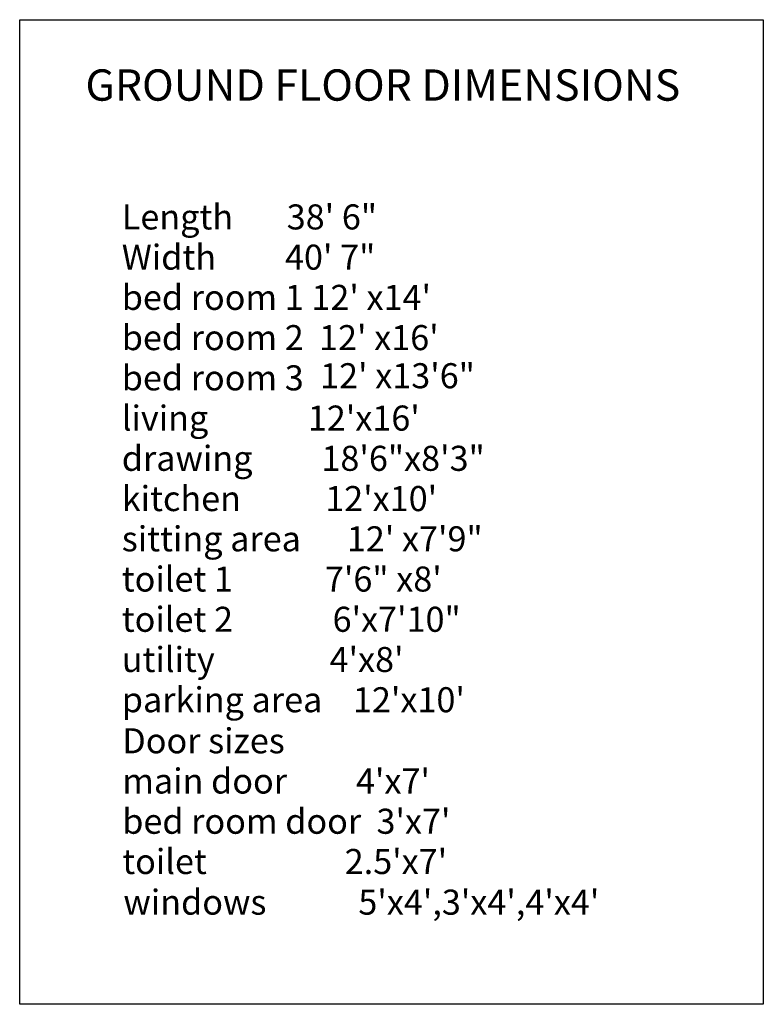
# Model space of a CAD drawing. Units: inches. Extents: x 2901 to 5923, y 918 to 2827.
# Tile 15 of 16: x 5128 to 5365, y 1343 to 1658. Entities that reach past the tile are written whole.
import ezdxf

# ---------------------------------------------------------------- set-up
doc = ezdxf.new("R2010")
doc.units = ezdxf.units.IN
doc.layers.add('A-ANNO-SCHD', color=7, linetype='Continuous', lineweight=25)
doc.layers.add('A-ANNO-TEXT', color=7, linetype='Continuous', lineweight=18)
doc.styles.get("Standard").update_dxf_attribs({"font": 'arial.ttf'})

msp = doc.modelspace()

# ---------------------------------------------------------------- linework, layer by layer
at = {"layer": 'A-ANNO-SCHD'}
msp.add_lwpolyline([(5127.94, 1657.97), (5365.27, 1657.97), (5365.27, 1343.49), (5127.94, 1343.49)], close=True, dxfattribs=at)

# ---------------------------------------------------------------- texts
at = {"layer": 'A-ANNO-TEXT'}
for s, height, p in [('GROUND FLOOR DIMENSIONS', 10, (5148.92, 1632.1)), ('Length       38\' 6"', 8, (5160.52, 1590.98)), ('Width         40\' 7"', 8, (5160.52, 1578.13)), ("bed room 1 12' x14'", 8, (5160.52, 1565.28)), ("bed room 2  12' x16'", 8, (5160.52, 1552.43)), ('bed room 3   ', 8, (5160.52, 1539.58)), ('   12\' x13\'6"', 8, (5216.48, 1540.26)), ("living             12'x16'", 8, (5160.52, 1526.73)), ('drawing         18\'6"x8\'3"', 8, (5160.52, 1513.88)), ("kitchen           12'x10'", 8, (5160.52, 1501.02)), ('sitting area      12\' x7\'9"', 8, (5160.52, 1488.17)), ('toilet 1            7\'6" x8\'', 8, (5160.52, 1475.32)), ('toilet 2             6\'x7\'10"', 8, (5160.52, 1462.47)), ("utility               4'x8'", 8, (5160.52, 1449.62)), ("parking area    12'x10'", 8, (5160.52, 1436.77)), ('Door sizes', 8, (5160.67, 1423.66)), ("main door         4'x7'", 8, (5160.67, 1410.81)), ("bed room door  3'x7'", 8, (5160.67, 1397.96)), ("toilet                  2.5'x7'", 8, (5160.67, 1385.11)), ("windows            5'x4',3'x4',4'x4'", 8, (5161.03, 1372.12))]:
    msp.add_text(s, height=height, dxfattribs=at).set_placement(p)

doc.saveas('drawing.dxf')
